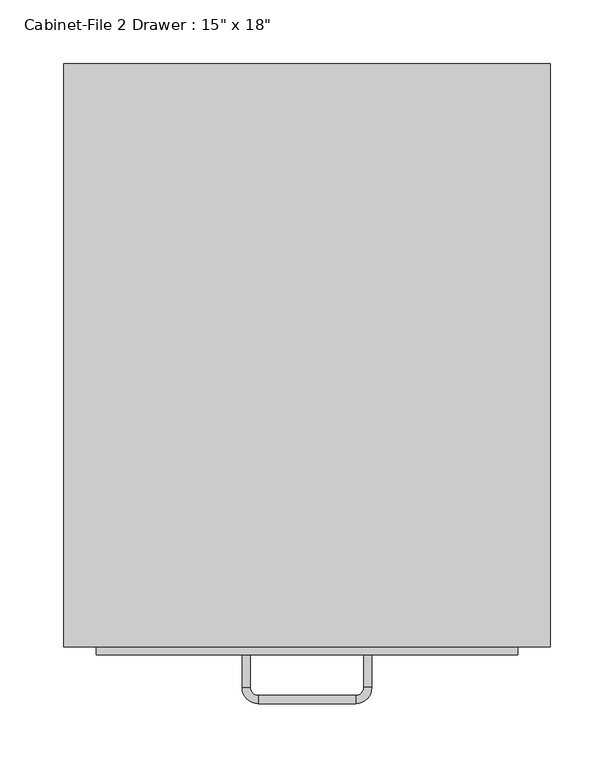
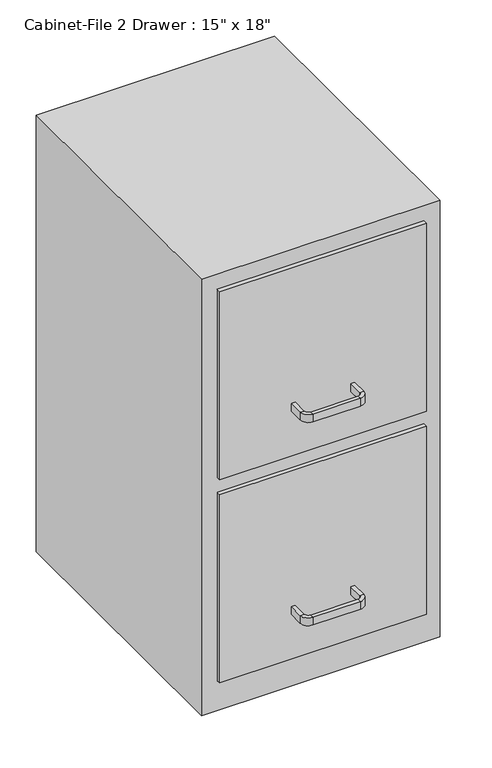
"""IFC4 building model written with IfcOpenShell, lengths in millimetres: furniture geometry."""

from ifc_helpers import new_model, si_unit, frame, origin, origin_with_axes, place, context, project, spatial, polyline, circle_curve, outline, extrude, source, transform, mapped, element, save
from ifc_brep_helpers import plane_surface, cylinder_surface, revolved_surface, advanced_brep


def furniture_bb55ed6b(model_context):
    return source(origin(), model_context, "Body", "SolidModel", [
        extrude(outline(polyline([(37.203553, -377.0843001), (-292.996447, -377.0843001), (-292.996447, -370.7343001), (37.203553, -370.7343001), (37.203553, -377.0843001)])), frame((0.0, 0.0, 393.7), z_axis=(0.0, 0.0, 1.0), x_axis=(1.0, 0.0, 0.0)), (0.0, 0.0, 1.0), 317.5),
        extrude(outline(polyline([(37.203553, -377.0843001), (-292.996447, -377.0843001), (-292.996447, -370.7343001), (37.203553, -370.7343001), (37.203553, -377.0843001)])), frame((0.0, 0.0, 50.8), z_axis=(0.0, 0.0, 1.0), x_axis=(1.0, 0.0, 0.0)), (0.0, 0.0, 1.0), 317.5),
        advanced_brep(
        [(-172.346447, -377.0843001, 127.0), (-178.696447, -377.0843001, 127.0), (-178.696447, -377.0843001, 139.7), (-172.346447, -377.0843001, 139.7), (-172.346447, -402.4843001, 127.0), (-178.696447, -402.4843001, 127.0), (-178.696447, -402.4843001, 139.7), (-172.346447, -402.4843001, 139.7), (-165.996447, -415.1843001, 127.0), (-165.996447, -408.8343001, 127.0), (-165.996447, -415.1843001, 139.7), (-165.996447, -408.8343001, 139.7), (-89.796447, -408.8343001, 127.0), (-89.796447, -415.1843001, 127.0), (-89.796447, -415.1843001, 139.7), (-89.796447, -408.8343001, 139.7), (-77.096447, -402.4843001, 127.0), (-83.446447, -402.4843001, 127.0), (-77.096447, -402.4843001, 139.7), (-83.446447, -402.4843001, 139.7), (-83.446447, -377.0843001, 127.0), (-83.446447, -377.0843001, 139.7), (-77.096447, -377.0843001, 139.7), (-77.096447, -377.0843001, 127.0)],
        [
            (0, 1),
            (1, 2),
            (2, 3),
            (3, 0),
            (0, 4),
            (4, 5),
            (5, 1),
            (5, 6),
            (6, 2),
            (6, 7),
            (7, 3),
            (7, 4),
            (8, 5, circle_curve(frame((-165.996447, -402.4843001, 127.0), z_axis=(0.0, 0.0, -1.0), x_axis=(-1.0, 0.0, 0.0)), 12.7)),
            (4, 9, circle_curve(frame((-165.996447, -402.4843001, 127.0), z_axis=(0.0, 0.0, 1.0), x_axis=(-1.0, 0.0, 0.0)), 6.35)),
            (9, 8),
            (10, 6, circle_curve(frame((-165.996447, -402.4843001, 139.7), z_axis=(0.0, 0.0, -1.0), x_axis=(-1.0, 0.0, 0.0)), 12.7)),
            (8, 10),
            (11, 7, circle_curve(frame((-165.996447, -402.4843001, 139.7), z_axis=(0.0, 0.0, -1.0), x_axis=(-1.0, 0.0, 0.0)), 6.35)),
            (10, 11),
            (11, 9),
            (9, 12),
            (12, 13),
            (13, 8),
            (13, 14),
            (14, 10),
            (14, 15),
            (15, 11),
            (15, 12),
            (16, 13, circle_curve(frame((-89.796447, -402.4843001, 127.0), z_axis=(0.0, 0.0, -1.0), x_axis=(0.0, -1.0, 0.0)), 12.7)),
            (12, 17, circle_curve(frame((-89.796447, -402.4843001, 127.0), z_axis=(0.0, 0.0, 1.0), x_axis=(0.0, -1.0, 0.0)), 6.35)),
            (17, 16),
            (18, 14, circle_curve(frame((-89.796447, -402.4843001, 139.7), z_axis=(0.0, 0.0, -1.0), x_axis=(0.0, -1.0, 0.0)), 12.7)),
            (16, 18),
            (19, 15, circle_curve(frame((-89.796447, -402.4843001, 139.7), z_axis=(0.0, 0.0, -1.0), x_axis=(0.0, -1.0, 0.0)), 6.35)),
            (18, 19),
            (19, 17),
            (20, 21),
            (21, 22),
            (22, 23),
            (23, 20),
            (17, 20),
            (23, 16),
            (22, 18),
            (21, 19),
        ],
        [
            plane_surface(frame((-661.3382215, -377.0843001, 0.0), z_axis=(0.0, 1.0, 0.0), x_axis=(0.0, 0.0, -1.0))),
            plane_surface(frame((-172.346447, -377.0843001, 127.0), z_axis=(0.0, 0.0, -1.0), x_axis=(0.0, -1.0, 0.0))),
            plane_surface(frame((-178.696447, -377.0843001, 127.0), z_axis=(-1.0, 0.0, 0.0), x_axis=(0.0, -1.0, 0.0))),
            plane_surface(frame((-178.696447, -377.0843001, 139.7), z_axis=(0.0, 0.0, 1.0), x_axis=(0.0, -1.0, 0.0))),
            plane_surface(frame((-172.346447, -377.0843001, 139.7), z_axis=(1.0, 0.0, 0.0), x_axis=(0.0, -1.0, 0.0))),
            plane_surface(frame((-165.996447, -402.4843001, 127.0), z_axis=(0.0, 0.0, -1.0), x_axis=(-1.0, 0.0, 0.0))),
            cylinder_surface(frame((-165.996447, -402.4843001, 0.0), z_axis=(0.0, 0.0, 1.0), x_axis=(-1.0, 0.0, 0.0)), 12.7),
            plane_surface(frame((-165.996447, -402.4843001, 139.7), z_axis=(0.0, 0.0, 1.0), x_axis=(-1.0, 0.0, 0.0))),
            revolved_surface(polyline([(-172.34644699999998, -402.4843001, 139.7), (-172.34644699999998, -402.4843001, 127.0)]), (-165.996447, -402.4843001, 0.0), (0.0, 0.0, 1.0)),
            plane_surface(frame((-165.996447, -408.8343001, 127.0), z_axis=(0.0, 0.0, -1.0), x_axis=(1.0, 0.0, 0.0))),
            plane_surface(frame((-165.996447, -415.1843001, 127.0), z_axis=(0.0, -1.0, 0.0), x_axis=(1.0, 0.0, 0.0))),
            plane_surface(frame((-165.996447, -415.1843001, 139.7), z_axis=(0.0, 0.0, 1.0), x_axis=(1.0, 0.0, 0.0))),
            plane_surface(frame((-165.996447, -408.8343001, 139.7), z_axis=(0.0, 1.0, 0.0), x_axis=(1.0, 0.0, 0.0))),
            plane_surface(frame((-89.796447, -402.4843001, 127.0), z_axis=(0.0, 0.0, -1.0), x_axis=(0.0, -1.0, 0.0))),
            cylinder_surface(frame((-89.796447, -402.4843001, 0.0), z_axis=(0.0, 0.0, 1.0), x_axis=(0.0, -1.0, 0.0)), 12.7),
            plane_surface(frame((-89.796447, -402.4843001, 139.7), z_axis=(0.0, 0.0, 1.0), x_axis=(0.0, -1.0, 0.0))),
            revolved_surface(polyline([(-89.796447, -408.8343001, 139.7), (-89.796447, -408.8343001, 127.0)]), (-89.796447, -402.4843001, 0.0), (0.0, 0.0, 1.0)),
            plane_surface(frame((-559.7382215, -377.0843001, 0.0), z_axis=(0.0, 1.0, 0.0), x_axis=(0.0, 0.0, 1.0))),
            plane_surface(frame((-83.446447, -402.4843001, 127.0), z_axis=(0.0, 0.0, -1.0), x_axis=(0.0, 1.0, 0.0))),
            plane_surface(frame((-77.096447, -402.4843001, 127.0), z_axis=(1.0, 0.0, 0.0), x_axis=(0.0, 1.0, 0.0))),
            plane_surface(frame((-77.096447, -402.4843001, 139.7), z_axis=(0.0, 0.0, 1.0), x_axis=(0.0, 1.0, 0.0))),
            plane_surface(frame((-83.446447, -402.4843001, 139.7), z_axis=(-1.0, 0.0, 0.0), x_axis=(0.0, 1.0, 0.0))),
        ],
        [
            (0, [[1, 2, 3, 4]]),
            (1, [[-1, 5, 6, 7]]),
            (2, [[-2, -7, 8, 9]]),
            (3, [[-3, -9, 10, 11]]),
            (4, [[-4, -11, 12, -5]]),
            (5, [[13, -6, 14, 15]]),
            (6, [[16, -8, -13, 17]]),
            (7, [[18, -10, -16, 19]]),
            (8, [[-14, -12, -18, 20]]),
            (9, [[-15, 21, 22, 23]]),
            (10, [[-17, -23, 24, 25]]),
            (11, [[-19, -25, 26, 27]]),
            (12, [[-20, -27, 28, -21]]),
            (13, [[29, -22, 30, 31]]),
            (14, [[32, -24, -29, 33]]),
            (15, [[34, -26, -32, 35]]),
            (16, [[-30, -28, -34, 36]]),
            (17, [[37, 38, 39, 40]]),
            (18, [[-31, 41, -40, 42]]),
            (19, [[-33, -42, -39, 43]]),
            (20, [[-35, -43, -38, 44]]),
            (21, [[-36, -44, -37, -41]]),
        ],
    ),
        advanced_brep(
        [(-172.346447, -377.0843001, 469.9), (-178.696447, -377.0843001, 469.9), (-178.696447, -377.0843001, 482.6), (-172.346447, -377.0843001, 482.6), (-172.346447, -402.4843001, 469.9), (-178.696447, -402.4843001, 469.9), (-178.696447, -402.4843001, 482.6), (-172.346447, -402.4843001, 482.6), (-165.996447, -415.1843001, 469.9), (-165.996447, -408.8343001, 469.9), (-165.996447, -415.1843001, 482.6), (-165.996447, -408.8343001, 482.6), (-89.796447, -408.8343001, 469.9), (-89.796447, -415.1843001, 469.9), (-89.796447, -415.1843001, 482.6), (-89.796447, -408.8343001, 482.6), (-77.096447, -402.4843001, 469.9), (-83.446447, -402.4843001, 469.9), (-77.096447, -402.4843001, 482.6), (-83.446447, -402.4843001, 482.6), (-83.446447, -377.0843001, 469.9), (-83.446447, -377.0843001, 482.6), (-77.096447, -377.0843001, 482.6), (-77.096447, -377.0843001, 469.9)],
        [
            (0, 1),
            (1, 2),
            (2, 3),
            (3, 0),
            (0, 4),
            (4, 5),
            (5, 1),
            (5, 6),
            (6, 2),
            (6, 7),
            (7, 3),
            (7, 4),
            (8, 5, circle_curve(frame((-165.996447, -402.4843001, 469.9), z_axis=(0.0, 0.0, -1.0), x_axis=(-1.0, 0.0, 0.0)), 12.7)),
            (4, 9, circle_curve(frame((-165.996447, -402.4843001, 469.9), z_axis=(0.0, 0.0, 1.0), x_axis=(-1.0, 0.0, 0.0)), 6.35)),
            (9, 8),
            (10, 6, circle_curve(frame((-165.996447, -402.4843001, 482.6), z_axis=(0.0, 0.0, -1.0), x_axis=(-1.0, 0.0, 0.0)), 12.7)),
            (8, 10),
            (11, 7, circle_curve(frame((-165.996447, -402.4843001, 482.6), z_axis=(0.0, 0.0, -1.0), x_axis=(-1.0, 0.0, 0.0)), 6.35)),
            (10, 11),
            (11, 9),
            (9, 12),
            (12, 13),
            (13, 8),
            (13, 14),
            (14, 10),
            (14, 15),
            (15, 11),
            (15, 12),
            (16, 13, circle_curve(frame((-89.796447, -402.4843001, 469.9), z_axis=(0.0, 0.0, -1.0), x_axis=(0.0, -1.0, 0.0)), 12.7)),
            (12, 17, circle_curve(frame((-89.796447, -402.4843001, 469.9), z_axis=(0.0, 0.0, 1.0), x_axis=(0.0, -1.0, 0.0)), 6.35)),
            (17, 16),
            (18, 14, circle_curve(frame((-89.796447, -402.4843001, 482.6), z_axis=(0.0, 0.0, -1.0), x_axis=(0.0, -1.0, 0.0)), 12.7)),
            (16, 18),
            (19, 15, circle_curve(frame((-89.796447, -402.4843001, 482.6), z_axis=(0.0, 0.0, -1.0), x_axis=(0.0, -1.0, 0.0)), 6.35)),
            (18, 19),
            (19, 17),
            (20, 21),
            (21, 22),
            (22, 23),
            (23, 20),
            (17, 20),
            (23, 16),
            (22, 18),
            (21, 19),
        ],
        [
            plane_surface(frame((-661.3382215, -377.0843001, 0.0), z_axis=(0.0, 1.0, 0.0), x_axis=(0.0, 0.0, -1.0))),
            plane_surface(frame((-172.346447, -377.0843001, 469.9), z_axis=(0.0, 0.0, -1.0), x_axis=(0.0, -1.0, 0.0))),
            plane_surface(frame((-178.696447, -377.0843001, 469.9), z_axis=(-1.0, 0.0, 0.0), x_axis=(0.0, -1.0, 0.0))),
            plane_surface(frame((-178.696447, -377.0843001, 482.6), z_axis=(0.0, 0.0, 1.0), x_axis=(0.0, -1.0, 0.0))),
            plane_surface(frame((-172.346447, -377.0843001, 482.6), z_axis=(1.0, 0.0, 0.0), x_axis=(0.0, -1.0, 0.0))),
            plane_surface(frame((-165.996447, -402.4843001, 469.9), z_axis=(0.0, 0.0, -1.0), x_axis=(-1.0, 0.0, 0.0))),
            cylinder_surface(frame((-165.996447, -402.4843001, 0.0), z_axis=(0.0, 0.0, 1.0), x_axis=(-1.0, 0.0, 0.0)), 12.7),
            plane_surface(frame((-165.996447, -402.4843001, 482.6), z_axis=(0.0, 0.0, 1.0), x_axis=(-1.0, 0.0, 0.0))),
            revolved_surface(polyline([(-172.34644699999998, -402.4843001, 482.6), (-172.34644699999998, -402.4843001, 469.9)]), (-165.996447, -402.4843001, 0.0), (0.0, 0.0, 1.0)),
            plane_surface(frame((-165.996447, -408.8343001, 469.9), z_axis=(0.0, 0.0, -1.0), x_axis=(1.0, 0.0, 0.0))),
            plane_surface(frame((-165.996447, -415.1843001, 469.9), z_axis=(0.0, -1.0, 0.0), x_axis=(1.0, 0.0, 0.0))),
            plane_surface(frame((-165.996447, -415.1843001, 482.6), z_axis=(0.0, 0.0, 1.0), x_axis=(1.0, 0.0, 0.0))),
            plane_surface(frame((-165.996447, -408.8343001, 482.6), z_axis=(0.0, 1.0, 0.0), x_axis=(1.0, 0.0, 0.0))),
            plane_surface(frame((-89.796447, -402.4843001, 469.9), z_axis=(0.0, 0.0, -1.0), x_axis=(0.0, -1.0, 0.0))),
            cylinder_surface(frame((-89.796447, -402.4843001, 0.0), z_axis=(0.0, 0.0, 1.0), x_axis=(0.0, -1.0, 0.0)), 12.7),
            plane_surface(frame((-89.796447, -402.4843001, 482.6), z_axis=(0.0, 0.0, 1.0), x_axis=(0.0, -1.0, 0.0))),
            revolved_surface(polyline([(-89.796447, -408.8343001, 482.6), (-89.796447, -408.8343001, 469.9)]), (-89.796447, -402.4843001, 0.0), (0.0, 0.0, 1.0)),
            plane_surface(frame((-559.7382215, -377.0843001, 0.0), z_axis=(0.0, 1.0, 0.0), x_axis=(0.0, 0.0, 1.0))),
            plane_surface(frame((-83.446447, -402.4843001, 469.9), z_axis=(0.0, 0.0, -1.0), x_axis=(0.0, 1.0, 0.0))),
            plane_surface(frame((-77.096447, -402.4843001, 469.9), z_axis=(1.0, 0.0, 0.0), x_axis=(0.0, 1.0, 0.0))),
            plane_surface(frame((-77.096447, -402.4843001, 482.6), z_axis=(0.0, 0.0, 1.0), x_axis=(0.0, 1.0, 0.0))),
            plane_surface(frame((-83.446447, -402.4843001, 482.6), z_axis=(-1.0, 0.0, 0.0), x_axis=(0.0, 1.0, 0.0))),
        ],
        [
            (0, [[1, 2, 3, 4]]),
            (1, [[-1, 5, 6, 7]]),
            (2, [[-2, -7, 8, 9]]),
            (3, [[-3, -9, 10, 11]]),
            (4, [[-4, -11, 12, -5]]),
            (5, [[13, -6, 14, 15]]),
            (6, [[16, -8, -13, 17]]),
            (7, [[18, -10, -16, 19]]),
            (8, [[-14, -12, -18, 20]]),
            (9, [[-15, 21, 22, 23]]),
            (10, [[-17, -23, 24, 25]]),
            (11, [[-19, -25, 26, 27]]),
            (12, [[-20, -27, 28, -21]]),
            (13, [[29, -22, 30, 31]]),
            (14, [[32, -24, -29, 33]]),
            (15, [[34, -26, -32, 35]]),
            (16, [[-30, -28, -34, 36]]),
            (17, [[37, 38, 39, 40]]),
            (18, [[-31, 41, -40, 42]]),
            (19, [[-33, -42, -39, 43]]),
            (20, [[-35, -43, -38, 44]]),
            (21, [[-36, -44, -37, -41]]),
        ],
    ),
        extrude(outline(polyline([(62.603553, 86.4656999), (62.603553, -370.7343001), (-318.396447, -370.7343001), (-318.396447, 86.4656999), (62.603553, 86.4656999)])), origin_with_axes(), (0.0, 0.0, 1.0), 736.6),
    ])


if __name__ == "__main__":
    model = new_model("IFC4")
    model_context = context("Model", 3, world=origin())
    ifc_project = project(units=[si_unit("LENGTHUNIT", "METRE", prefix="MILLI")], contexts=[model_context])
    site = spatial("IfcSite", under=ifc_project)
    building = spatial("IfcBuilding", under=site)
    placement = place(None, origin())
    furniture_shape = furniture_bb55ed6b(model_context)
    element("IfcFurniture", 1, ObjectType="Cabinet-File 2 Drawer : 15\" x 18\"", at=placement, inside=building, context=model_context, shape_type="MappedRepresentation", body=[
        mapped(furniture_shape, transform((0.0, 0.0, 0.0), x_axis=(1.0, 0.0, 0.0), y_axis=(0.0, 1.0, 0.0), z_axis=(0.0, 0.0, 1.0))),
    ])
    save(model, "model.ifc")

# Revit data of these elements
# Type "Cabinet-File 2 Drawer : 15\" x 18\""
#   Assembly Code = "E2020200"
#   Depth = 1' - 6"
#   Height = 2' - 5"
#   Width = 1' - 3"
#   Cabinet Material = Wood - Teak
#   Handle Material = Steel, Chrome Plated
#   Default Elevation = 0
# Element 1 (IfcFurniture, "Cabinet-File 2 Drawer : 15\" x 18\"")
#   Materials on its faces: "Steel, Chrome Plated", "Wood - Teak"
# Materials
#   "Wood - Teak": class "Wood", colour RGB 145 112 90, transparency 0
#   "Steel, Chrome Plated": class "Metal", colour RGB 17 17 17, transparency 0, Description = "Chromiuim plated steel", Cost = 0
